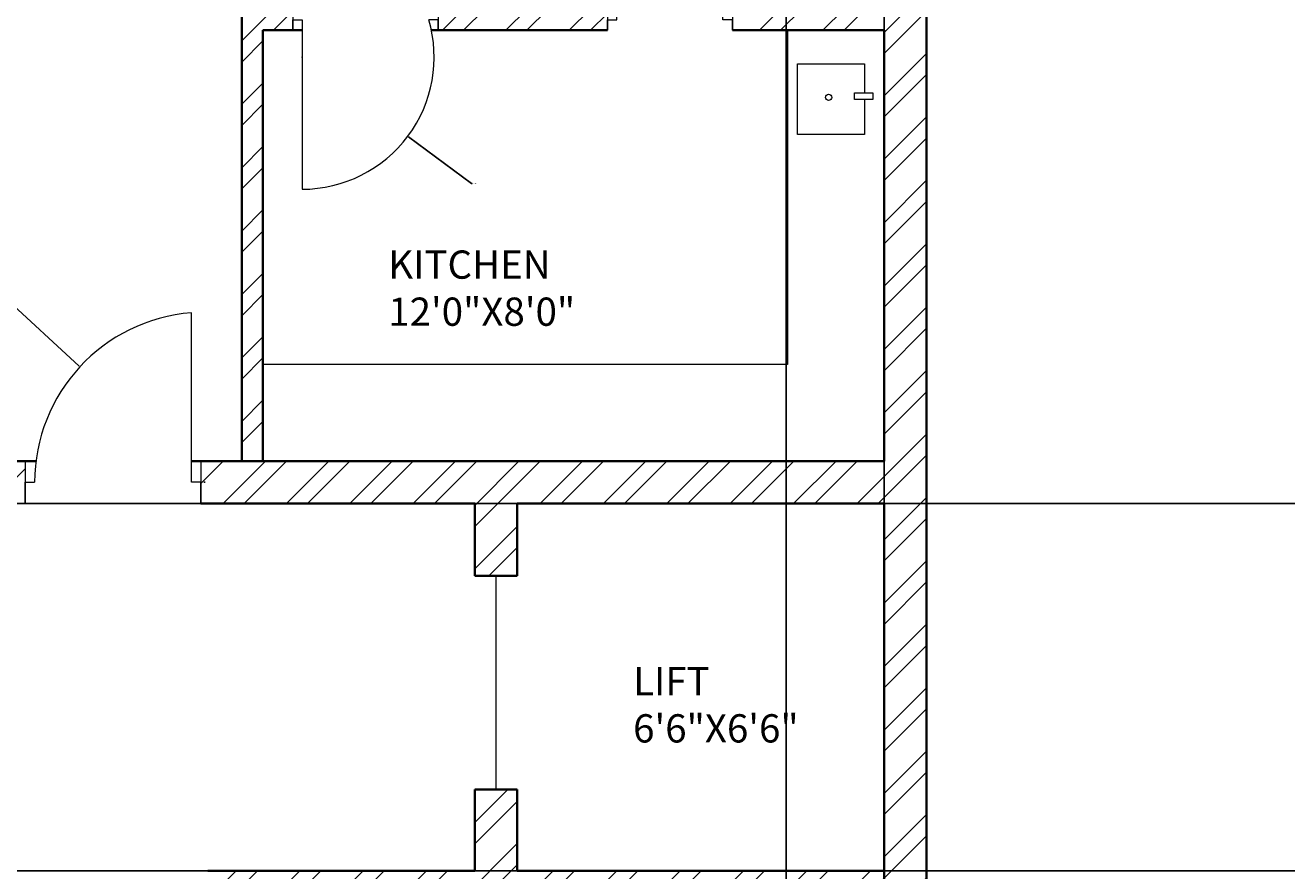
# Model space of a CAD drawing. Units: inches. Extents: x 1355 to 2746, y 1171 to 2751.
# Tile 11 of 24: x 1749 to 2017, y 1686 to 1866. Entities that reach past the tile are written whole.
import ezdxf

# ---------------------------------------------------------------- set-up
doc = ezdxf.new("R2010")
doc.units = ezdxf.units.IN
for name, color, linetype, lineweight in [('A-ANNO-DIMS', 2, 'Continuous', 18), ('A-AREA-IDEN', 7, 'Continuous', 18), ('A-DOOR', 3, 'Continuous', 20), ('A-FLOR-CASE', 30, 'Continuous', 20), ('A-FLOR-FIXT', 9, 'Continuous', 18), ('A-WALL', 7, 'Continuous', 40), ('A-WALL-PATT', 252, 'Continuous', 13)]:
    doc.layers.add(name, color=color, linetype=linetype, lineweight=lineweight)
doc.styles.get("Standard").update_dxf_attribs({"font": 'arial.ttf'})
doc.dimstyles.get("Standard").update_dxf_attribs({"dimtxt": 0.18, "dimasz": 0.18, "dimexe": 0.18, "dimexo": 0.0625, "dimgap": 0.09, "dimtad": 0, "dimtih": 1, "dimtoh": 1, "dimdec": 4, "dimzin": 0, "dimdsep": 46, "dimtxsty": 'Standard', "dimcen": 0.09, "dimadec": 0, "dimazin": 0, "dimtfac": 1, "dimtdec": 4, "dimtofl": 0, "dimtmove": 0, "dimatfit": 3, "dimfxl": 1, "dimtolj": 1, "dimtzin": 0, "dimarcsym": 0})

# ---------------------------------------------------------------- blocks, each defined once
blk = doc.blocks.new('DOOR-ENTRY-N')
for p, q in [((35.29, 4.5), (35.29, 40.5)), ((0, 9), (0, 0)), ((37.29, 9), (37.29, 0)), ((0, 0), (0, 4.5)), ((0, 4.5), (2, 4.5)), ((37.29, 4.5), (35.29, 4.5)), ((37.29, 0), (37.29, 4.5))]:
    blk.add_line(p, q)
blk.add_arc((38.11, 4.5), 36.11, 94.4716, 180)
blk = doc.blocks.new('DOOR-UTILITY-N')
for p, q in [((2, 2.25), (2, 26.25)), ((0, 4.5), (0, 0)), ((26.56, 4.5), (26.56, 0)), ((0, 0), (0, 2.25)), ((0, 2.25), (2, 2.25)), ((26.56, 2.25), (24.56, 2.25)), ((26.56, 0), (26.56, 2.25))]:
    blk.add_line(p, q)
blk.add_arc((0.51, 2.25), 24.05, 0, 86.4557)
blk = doc.blocks.new('DOOR-KITCHEN-N')
for p, q in [((0, 38.25), (0, 33.75)), ((30.9, 38.25), (30.9, 33.75)), ((0, 33.75), (0, 36)), ((0, 36), (2, 36)), ((2, 36), (2, 0)), ((30.9, 36), (28.9, 36)), ((30.9, 33.75), (30.9, 36))]:
    blk.add_line(p, q)
blk.add_arc((2, 28.05), 28.05, 270, 16.4594)
blk = doc.blocks.new('*D102')
at = {"layer": 'A-ANNO-DIMS', "color": 0, "lineweight": -2, "transparency": 16777216}
for p, q in [((2089.33, 1764.3), (1407.53, 1764.3)), ((1407.71, 1764.12), (1407.71, 1725.48)), ((1407.71, 1686.48), (1407.71, 1725.12)), ((2089.33, 1686.3), (1407.53, 1686.3))]:
    blk.add_line(p, q, dxfattribs=at)
at = {"layer": 'A-ANNO-DIMS', "color": 0, "transparency": 16777216}
for points in [[(1407.68, 1764.12), (1407.74, 1764.12), (1407.71, 1764.3)], [(1407.68, 1686.48), (1407.74, 1686.48), (1407.71, 1686.3)]]:
    blk.add_solid(points, dxfattribs=at)
at = {"layer": 'Defpoints', "color": 0, "transparency": 16777216}
for p in [(1407.71, 1764.3), (2089.39, 1764.3), (2089.39, 1686.3)]:
    blk.add_point(p, dxfattribs=at)
at = {"layer": 'A-ANNO-DIMS', "color": 0, "transparency": 16777216, "insert": (1407.71, 1725.3), "char_height": 0.18, "attachment_point": 5}
blk.add_mtext('\\A1;78', dxfattribs=at)
blk = doc.blocks.new('*D103')
at = {"layer": 'A-ANNO-DIMS', "color": 0, "lineweight": -2, "transparency": 16777216}
for p, q in [((2089.33, 1917.3), (1407.53, 1917.3)), ((1407.71, 1917.12), (1407.71, 1840.98)), ((1407.71, 1764.48), (1407.71, 1840.62)), ((2089.33, 1764.3), (1407.53, 1764.3))]:
    blk.add_line(p, q, dxfattribs=at)
at = {"layer": 'A-ANNO-DIMS', "color": 0, "transparency": 16777216}
for points in [[(1407.68, 1917.12), (1407.74, 1917.12), (1407.71, 1917.3)], [(1407.68, 1764.48), (1407.74, 1764.48), (1407.71, 1764.3)]]:
    blk.add_solid(points, dxfattribs=at)
at = {"layer": 'Defpoints', "color": 0, "transparency": 16777216}
for p in [(1407.71, 1917.3), (2089.39, 1917.3), (2089.39, 1764.3)]:
    blk.add_point(p, dxfattribs=at)
at = {"layer": 'A-ANNO-DIMS', "color": 0, "transparency": 16777216, "insert": (1407.71, 1840.8), "char_height": 0.18, "attachment_point": 5}
blk.add_mtext('\\A1;153', dxfattribs=at)
blk = doc.blocks.new('*D107')
at = {"layer": 'A-ANNO-DIMS', "color": 0, "lineweight": -2, "transparency": 16777216}
for p, q in [((2089.33, 1686.3), (1407.53, 1686.3)), ((1407.71, 1686.12), (1407.71, 1622.26)), ((1407.71, 1558.03), (1407.71, 1621.89)), ((2031.09, 1557.85), (1407.53, 1557.85))]:
    blk.add_line(p, q, dxfattribs=at)
at = {"layer": 'A-ANNO-DIMS', "color": 0, "transparency": 16777216}
for points in [[(1407.68, 1686.12), (1407.74, 1686.12), (1407.71, 1686.3)], [(1407.68, 1558.03), (1407.74, 1558.03), (1407.71, 1557.85)]]:
    blk.add_solid(points, dxfattribs=at)
at = {"layer": 'Defpoints', "color": 0, "transparency": 16777216}
for p in [(1407.71, 1686.3), (2089.39, 1686.3), (2031.15, 1557.85)]:
    blk.add_point(p, dxfattribs=at)
at = {"layer": 'A-ANNO-DIMS', "color": 0, "transparency": 16777216, "insert": (1407.71, 1622.07), "char_height": 0.18, "attachment_point": 5}
blk.add_mtext('\\A1;128.46', dxfattribs=at)
blk = doc.blocks.new('*D145')
at = {"layer": 'A-ANNO-DIMS', "color": 0, "lineweight": -2, "transparency": 16777216}
for p, q in [((1910.88, 1399.86), (1910.88, 2716.58)), ((1911.06, 2716.4), (1920.83, 2716.4)), ((1931.53, 2716.4), (1921.76, 2716.4)), ((1931.71, 1399.86), (1931.71, 2716.58))]:
    blk.add_line(p, q, dxfattribs=at)
at = {"layer": 'A-ANNO-DIMS', "color": 0, "transparency": 16777216}
for points in [[(1911.06, 2716.43), (1911.06, 2716.37), (1910.88, 2716.4)], [(1931.53, 2716.43), (1931.53, 2716.37), (1931.71, 2716.4)]]:
    blk.add_solid(points, dxfattribs=at)
at = {"layer": 'Defpoints', "color": 0, "transparency": 16777216}
for p in [(1931.71, 2716.4), (1910.88, 1399.8), (1931.71, 1399.8)]:
    blk.add_point(p, dxfattribs=at)
at = {"layer": 'A-ANNO-DIMS', "color": 0, "transparency": 16777216, "insert": (1921.3, 2716.4), "char_height": 0.18, "attachment_point": 5}
blk.add_mtext('\\A1;20.824', dxfattribs=at)
blk = doc.blocks.new('*D154')
at = {"layer": 'A-ANNO-DIMS', "color": 0, "lineweight": -2, "transparency": 16777216}
for p, q in [((1744.73, 1808.03), (1744.91, 1808.03)), ((1744.91, 1808.03), (1760.69, 1793.44)), ((1787.24, 1768.8), (1787.42, 1768.8)), ((1787.33, 1768.71), (1787.33, 1768.89))]:
    blk.add_line(p, q, dxfattribs=at)
at = {"layer": 'A-ANNO-DIMS', "color": 0, "transparency": 16777216}
blk.add_solid([(1760.71, 1793.46), (1760.67, 1793.42), (1760.82, 1793.32)], dxfattribs=at)
at = {"layer": 'Defpoints', "color": 0, "transparency": 16777216}
for p in [(1760.82, 1793.32), (1787.33, 1768.8)]:
    blk.add_point(p, dxfattribs=at)
at = {"layer": 'A-ANNO-DIMS', "color": 0, "transparency": 16777216, "insert": (1744.27, 1808.03), "char_height": 0.18, "attachment_point": 5}
blk.add_mtext('\\A1;R36.11', dxfattribs=at)
blk = doc.blocks.new('*D158')
at = {"layer": 'A-ANNO-DIMS', "color": 0, "lineweight": -2, "transparency": 16777216}
for p, q in [((1807.96, 1859.1), (1808.14, 1859.1)), ((1808.05, 1859.01), (1808.05, 1859.19)), ((1844.01, 1832.24), (1830.67, 1842.2)), ((1844.19, 1832.24), (1844.01, 1832.24))]:
    blk.add_line(p, q, dxfattribs=at)
at = {"layer": 'A-ANNO-DIMS', "color": 0, "transparency": 16777216}
blk.add_solid([(1830.69, 1842.23), (1830.65, 1842.18), (1830.52, 1842.31)], dxfattribs=at)
at = {"layer": 'Defpoints', "color": 0, "transparency": 16777216}
for p in [(1808.05, 1859.1), (1830.52, 1842.31)]:
    blk.add_point(p, dxfattribs=at)
at = {"layer": 'A-ANNO-DIMS', "color": 0, "transparency": 16777216, "insert": (1844.67, 1832.24), "char_height": 0.18, "attachment_point": 5}
blk.add_mtext('\\A1;R28.05', dxfattribs=at)

msp = doc.modelspace()

# ---------------------------------------------------------------- hatches: boundary and pattern name
at = {"layer": 'A-WALL-PATT'}
h = msp.add_hatch(dxfattribs=at)
h.set_pattern_fill('ANSI32', color=256)
h.paths.add_polyline_path([(1660.2083, 2139.3018), (1614.5977, 2139.3018), (1614.5977, 2130.3018), (1655.7083, 2130.3018), (1655.7083, 1981.8018), (1660.2083, 1981.8018), (1660.2083, 2090.7225), (1692.5832, 2090.7225), (1692.5832, 2095.2225), (1660.2083, 2095.2225)])
h.paths.add_polyline_path([(1523.7083, 2130.3018), (1554.5977, 2130.3018), (1554.5977, 2134.8018), (1554.5977, 2139.3018), (1514.7083, 2139.3018), (1514.7083, 2071.8385), (1523.7083, 2071.8385)])
h.paths.add_polyline_path([(1940.7083, 2139.3018), (1883.7928, 2139.3018), (1883.7928, 2130.3018), (1931.7083, 2130.3018), (1931.7083, 2098.3333), (1940.7083, 2098.3333)])
h.paths.add_polyline_path([(1799.7083, 2130.3018), (1823.7928, 2130.3018), (1823.7928, 2134.8018), (1823.7928, 2139.3018), (1795.2083, 2139.3018), (1795.2083, 2130.3018), (1795.2083, 2095.2225), (1759.2134, 2095.2225), (1759.2134, 2090.7225), (1795.2083, 2090.7225), (1795.2083, 1981.8018), (1799.7083, 1981.8018), (1799.7083, 1986.3018)])
h.paths.add_polyline_path([(1940.7083, 2038.3333), (1931.7083, 2038.3333), (1931.7083, 1986.3018), (1832.7083, 1986.3018), (1832.7083, 1947.1338), (1837.2083, 1947.1338), (1837.2083, 1981.8018), (1931.7083, 1981.8018), (1931.7083, 1967.1939), (1940.7083, 1967.1939)])
h.paths.add_polyline_path([(1940.7083, 1943.1939), (1931.7083, 1943.1939), (1931.7083, 1921.8018), (1837.2083, 1921.8018), (1837.2083, 1926.0511), (1832.7083, 1926.0511), (1832.7083, 1917.3018), (1931.7083, 1917.3018), (1931.7083, 1908.3321), (1940.7083, 1908.3321)])
h.paths.add_polyline_path([(1940.7083, 1884.3321), (1931.7083, 1884.3321), (1931.7083, 1869.3018), (1899.4583, 1869.3018), (1899.4583, 1864.8018), (1931.7083, 1864.8018), (1931.7083, 1773.3018), (1786.5143, 1773.3018), (1786.5143, 1764.3018), (1844.7083, 1764.3018), (1844.7083, 1748.9343), (1853.7083, 1748.9343), (1853.7083, 1764.3018), (1931.7083, 1764.3018), (1931.7083, 1652.9424), (1940.7083, 1652.9424)])
h.paths.add_polyline_path([(1799.7083, 1864.8018), (1806.0522, 1864.8018), (1806.0522, 1867.0518), (1806.0522, 1869.3018), (1799.7083, 1869.3018), (1799.7083, 1917.3018), (1799.7083, 1921.8018), (1795.2083, 1921.8018), (1795.2083, 1773.3018), (1799.7083, 1773.3018)])
h.paths.add_polyline_path([(1872.8988, 1867.0518), (1872.8988, 1869.3018), (1867.2083, 1869.3018), (1867.2083, 1917.3018), (1862.7083, 1917.3018), (1862.7083, 1869.3018), (1836.9546, 1869.3018), (1836.9546, 1864.8018), (1862.7083, 1864.8018), (1872.8988, 1864.8018)])
h.paths.add_polyline_path([(1749.2197, 1773.3018), (1655.7083, 1773.3018), (1523.7083, 1773.3018), (1523.7083, 1828.4963), (1514.7083, 1828.4963), (1514.7083, 1753.9033), (1519.2083, 1753.9033), (1523.7083, 1753.9033), (1523.7083, 1764.3018), (1655.7083, 1764.3018), (1749.2197, 1764.3018), (1749.2197, 1768.8018)])
h.paths.add_polyline_path([(1660.2083, 1921.8018), (1655.7083, 1921.8018), (1655.7083, 1917.3018), (1655.7083, 1773.3018), (1660.2083, 1773.3018)])
h.paths.add_polyline_path([(1523.7083, 2011.8385), (1514.7083, 2011.8385), (1514.7083, 1973.114), (1519.2083, 1973.114), (1523.7083, 1973.114), (1523.7083, 1976.8227), (1523.7083, 1981.8018), (1618.2083, 1981.8018), (1618.2083, 1921.8018), (1553.707, 1921.8018), (1553.707, 1917.3018), (1622.7083, 1917.3018), (1622.7083, 1919.5518), (1622.7083, 1921.8018), (1622.7083, 1986.3018), (1523.7083, 1986.3018)])
h.paths.add_polyline_path([(1529.6686, 1919.5518), (1529.6686, 1921.8018), (1523.7083, 1921.8018), (1523.7083, 1949.114), (1514.7083, 1949.114), (1514.7083, 1888.4963), (1523.7083, 1888.4963), (1523.7083, 1917.3018), (1529.6686, 1917.3018)])
h.paths.add_polyline_path([(1538.9419, 1775.643), (1585.5504, 1775.643), (1585.5504, 1798.0318), (1538.9419, 1798.0318)], flags=25)
h.paths.add_polyline_path([(1696.7097, 1497.3356), (1769.5651, 1497.3356), (1769.5651, 1523.4559), (1696.7097, 1523.4559)], flags=9)
h.paths.add_polyline_path([(1629.1643, 1230.5133), (1877.0879, 1230.5133), (1877.0879, 1267.606), (1629.1643, 1267.606)], flags=9)
h.paths.add_polyline_path([(2533.4462, 2215.4033), (2579.9292, 2215.4033), (2579.9292, 2231.889), (2533.4462, 2231.889)], flags=9)
h.paths.add_polyline_path([(2540.822, 2515.6945), (2594.2245, 2515.6945), (2594.2245, 2545.5463), (2540.822, 2545.5463)], flags=9)
h.paths.add_polyline_path([(2535.9857, 2588.2819), (2582.4687, 2588.2819), (2582.4687, 2604.7675), (2535.9857, 2604.7675)], flags=9)
h.paths.add_polyline_path([(2537.1627, 2617.1172), (2649.1245, 2617.1172), (2649.1245, 2633.6029), (2537.1627, 2633.6029)], flags=9)
h.paths.add_polyline_path([(2218.0051, 2168.228), (2363.9573, 2168.228), (2363.9573, 2205.3208), (2218.0051, 2205.3208)], flags=9)
h.paths.add_polyline_path([(1650.2156, 2165.3631), (1800.3547, 2165.3631), (1800.3547, 2202.4559), (1650.2156, 2202.4559)], flags=9)
h.paths.add_polyline_path([(2553.9592, 1610.7663), (2588.4203, 1610.7663), (2588.4203, 1660.2233), (2553.9592, 1660.2233)], flags=9)
h.paths.add_polyline_path([(1549.0868, 1648.2033), (1595.6952, 1648.2033), (1595.6952, 1670.5921), (1549.0868, 1670.5921)], flags=9)
h.paths.add_polyline_path([(1546.9525, 1502.0931), (1583.3413, 1502.0931), (1583.3413, 1524.4819), (1546.9525, 1524.4819)], flags=9)
h.paths.add_polyline_path([(1540.7704, 1433.4431), (1587.3788, 1433.4431), (1587.3788, 1455.8319), (1540.7704, 1455.8319)], flags=9)
h.paths.add_polyline_path([(1683.6524, 1321.5269), (1760.6169, 1321.5269), (1760.6169, 1333.8911), (1683.6524, 1333.8911)], flags=9)
h.paths.add_polyline_path([(1832.0485, 1356.0874), (1873.0989, 1356.0874), (1873.0989, 1378.4762), (1832.0485, 1378.4762)], flags=9)
h.paths.add_polyline_path([(1877.9694, 1431.2138), (1926.3827, 1431.2138), (1926.3827, 1453.578), (1877.9694, 1453.578)], flags=9)
h.paths.add_polyline_path([(1847.3106, 1499.8371), (1883.6994, 1499.8371), (1883.6994, 1522.2259), (1847.3106, 1522.2259)], flags=9)
h.paths.add_polyline_path([(1813.7015, 1640.7287), (1860.3099, 1640.7287), (1860.3099, 1663.1175), (1813.7015, 1663.1175)], flags=9)
h.paths.add_polyline_path([(1876.2576, 1710.2471), (1912.9452, 1710.2471), (1912.9452, 1732.6359), (1876.2576, 1732.6359)], flags=25)
h.paths.add_polyline_path([(1695.9163, 1715.3064), (1736.9668, 1715.3064), (1736.9668, 1737.6952), (1695.9163, 1737.6952)], flags=9)
h.paths.add_polyline_path([(1881.8583, 1888.9094), (1930.2717, 1888.9094), (1930.2717, 1911.2737), (1881.8583, 1911.2737)], flags=9)
h.paths.add_polyline_path([(1823.9298, 1798.6431), (1864.9803, 1798.6431), (1864.9803, 1821.0319), (1823.9298, 1821.0319)], flags=25)
h.paths.add_polyline_path([(1845.6062, 1948.1408), (1881.995, 1948.1408), (1881.995, 1970.5296), (1845.6062, 1970.5296)], flags=25)
h.paths.add_polyline_path([(1849.027, 1991.5151), (1895.6355, 1991.5151), (1895.6355, 2013.9039), (1849.027, 2013.9039)], flags=25)
h.paths.add_polyline_path([(1684.9725, 2113.8416), (1764.2658, 2113.8416), (1764.2658, 2126.2058), (1684.9725, 2126.2058)], flags=9)
h.paths.add_polyline_path([(1688.6193, 1913.0676), (1776.2005, 1913.0676), (1776.2005, 1935.4564), (1688.6193, 1935.4564)], flags=9)
h.paths.add_polyline_path([(1571.4689, 1930.9816), (1607.8577, 1930.9816), (1607.8577, 1953.3704), (1571.4689, 1953.3704)], flags=25)
h.paths.add_polyline_path([(1535.3581, 1998.3125), (1581.9665, 1998.3125), (1581.9665, 2020.7014), (1535.3581, 2020.7014)], flags=9)
h = msp.add_hatch(dxfattribs=at)
h.set_pattern_fill('ANSI32', color=256)
h.paths.add_polyline_path([(1749.2197, 1686.3018), (1732.6892, 1686.3018), (1523.7083, 1686.3018), (1523.7083, 1705.9033), (1514.7083, 1705.9033), (1514.7083, 1647.8732), (1519.2083, 1647.8732), (1523.7083, 1647.8732), (1523.7083, 1677.3018), (1655.7083, 1677.3018), (1655.7083, 1528.8018), (1660.2083, 1528.8018), (1660.2083, 1677.3018), (1732.6892, 1677.3018), (1749.2197, 1677.3018)])
h.paths.add_polyline_path([(1931.7083, 1686.3018), (1853.7083, 1686.3018), (1853.7083, 1703.5696), (1844.7083, 1703.5696), (1844.7083, 1686.3018), (1788.0274, 1686.3018), (1788.0274, 1677.3018), (1795.2083, 1677.3018), (1795.2083, 1528.8018), (1799.7083, 1528.8018), (1799.7083, 1677.3018), (1844.7083, 1677.3018), (1931.7083, 1677.3018)])
h.paths.add_polyline_path([(1931.7083, 1533.3018), (1844.7083, 1533.3018), (1832.7083, 1533.3018), (1832.7083, 1531.0518), (1832.7083, 1528.8018), (1832.7083, 1495.7519), (1837.2083, 1495.7519), (1837.2083, 1528.8018), (1931.7083, 1528.8018)])
h.paths.add_polyline_path([(1940.7083, 1592.9424), (1931.7083, 1592.9424), (1931.7083, 1506.7845), (1940.7083, 1506.7845)])
h.paths.add_polyline_path([(1940.7083, 1482.7845), (1936.2083, 1482.7845), (1931.7083, 1482.7845), (1931.7083, 1320.3018), (1880.7083, 1320.3018), (1880.7083, 1311.3018), (1940.7083, 1311.3018)])
h.paths.add_polyline_path([(1931.7083, 1468.8018), (1844.7083, 1468.8018), (1837.2083, 1468.8018), (1837.2083, 1474.34), (1832.7083, 1474.34), (1832.7083, 1468.8018), (1832.7083, 1464.3018), (1844.7083, 1464.3018), (1931.7083, 1464.3018)])
h.paths.add_polyline_path([(1863.8571, 1464.3018), (1859.3571, 1464.3018), (1859.3571, 1404.1662), (1838.1542, 1404.1662), (1838.1542, 1399.8018), (1869.4185, 1399.8018), (1869.4185, 1402.0518), (1869.4185, 1404.3018), (1863.8571, 1404.3018)])
h.paths.add_polyline_path([(1799.7083, 1399.6662), (1805.4082, 1399.6662), (1805.4082, 1401.9162), (1805.4082, 1404.1662), (1799.7083, 1404.1662), (1799.7083, 1464.3018), (1799.7083, 1468.8018), (1795.2083, 1468.8018), (1795.2083, 1356.2098), (1761.2597, 1356.2098), (1761.2597, 1351.7098), (1795.2083, 1351.7098), (1795.2083, 1320.3018), (1795.2083, 1311.3018), (1844.7083, 1311.3018), (1844.7083, 1315.8018), (1844.7083, 1320.3018), (1799.7083, 1320.3018)])
h.paths.add_polyline_path([(1692.9218, 1356.2098), (1660.2083, 1356.2098), (1660.2083, 1430.786), (1657.9583, 1430.786), (1655.7083, 1430.786), (1655.7083, 1320.3018), (1611.934, 1320.3018), (1611.934, 1311.3018), (1660.2083, 1311.3018), (1660.2083, 1351.7098), (1692.9218, 1351.7098)])
h.paths.add_polyline_path([(1523.7083, 1372.653), (1514.7083, 1372.653), (1514.7083, 1311.3018), (1551.934, 1311.3018), (1551.934, 1315.8018), (1551.934, 1320.3018), (1523.7083, 1320.3018)])
h.paths.add_polyline_path([(1523.7083, 1490.9023), (1514.7083, 1490.9023), (1514.7083, 1432.653), (1519.2083, 1432.653), (1523.7083, 1432.653)])
h.paths.add_polyline_path([(1660.2083, 1468.8018), (1622.7083, 1468.8018), (1622.7083, 1473.1566), (1618.2083, 1473.1566), (1618.2083, 1468.8018), (1523.7083, 1468.8018), (1523.7083, 1464.3018), (1655.7083, 1464.3018), (1655.7083, 1460.5634), (1660.2083, 1460.5634)])
h.paths.add_polyline_path([(1523.7083, 1587.8732), (1514.7083, 1587.8732), (1514.7083, 1514.9023), (1519.2083, 1514.9023), (1523.7083, 1514.9023)])
h.paths.add_polyline_path([(1622.7083, 1533.3018), (1523.7083, 1533.3018), (1523.7083, 1528.8018), (1618.2083, 1528.8018), (1618.2083, 1494.4205), (1622.7083, 1494.4205), (1622.7083, 1528.8018)])
h.paths.add_polyline_path([(1696.7097, 1497.3356), (1769.5651, 1497.3356), (1769.5651, 1523.4559), (1696.7097, 1523.4559)], flags=9)
h.paths.add_polyline_path([(1629.1643, 1230.5133), (1877.0879, 1230.5133), (1877.0879, 1267.606), (1629.1643, 1267.606)], flags=9)
h.paths.add_polyline_path([(2533.4462, 2215.4033), (2579.9292, 2215.4033), (2579.9292, 2231.889), (2533.4462, 2231.889)], flags=9)
h.paths.add_polyline_path([(2540.822, 2515.6945), (2594.2245, 2515.6945), (2594.2245, 2545.5463), (2540.822, 2545.5463)], flags=9)
h.paths.add_polyline_path([(2535.9857, 2588.2819), (2582.4687, 2588.2819), (2582.4687, 2604.7675), (2535.9857, 2604.7675)], flags=9)
h.paths.add_polyline_path([(2537.1627, 2617.1172), (2649.1245, 2617.1172), (2649.1245, 2633.6029), (2537.1627, 2633.6029)], flags=9)
h.paths.add_polyline_path([(2218.0051, 2168.228), (2363.9573, 2168.228), (2363.9573, 2205.3208), (2218.0051, 2205.3208)], flags=9)
h.paths.add_polyline_path([(1650.2156, 2165.3631), (1800.3547, 2165.3631), (1800.3547, 2202.4559), (1650.2156, 2202.4559)], flags=9)
h.paths.add_polyline_path([(2553.9592, 1610.7663), (2588.4203, 1610.7663), (2588.4203, 1660.2233), (2553.9592, 1660.2233)], flags=9)
h.paths.add_polyline_path([(1549.0868, 1648.2033), (1595.6952, 1648.2033), (1595.6952, 1670.5921), (1549.0868, 1670.5921)], flags=25)
h.paths.add_polyline_path([(1546.9525, 1502.0931), (1583.3413, 1502.0931), (1583.3413, 1524.4819), (1546.9525, 1524.4819)], flags=25)
h.paths.add_polyline_path([(1540.7704, 1433.4431), (1587.3788, 1433.4431), (1587.3788, 1455.8319), (1540.7704, 1455.8319)], flags=9)
h.paths.add_polyline_path([(1683.6524, 1321.5269), (1760.6169, 1321.5269), (1760.6169, 1333.8911), (1683.6524, 1333.8911)], flags=9)
h.paths.add_polyline_path([(1832.0485, 1356.0874), (1873.0989, 1356.0874), (1873.0989, 1378.4762), (1832.0485, 1378.4762)], flags=9)
h.paths.add_polyline_path([(1877.9694, 1431.2138), (1926.3827, 1431.2138), (1926.3827, 1453.578), (1877.9694, 1453.578)], flags=9)
h.paths.add_polyline_path([(1847.3106, 1499.8371), (1883.6994, 1499.8371), (1883.6994, 1522.2259), (1847.3106, 1522.2259)], flags=25)
h.paths.add_polyline_path([(1813.7015, 1640.7287), (1860.3099, 1640.7287), (1860.3099, 1663.1175), (1813.7015, 1663.1175)], flags=25)
h.paths.add_polyline_path([(1876.2576, 1710.2471), (1912.9452, 1710.2471), (1912.9452, 1732.6359), (1876.2576, 1732.6359)], flags=9)
h.paths.add_polyline_path([(1695.9163, 1715.3064), (1736.9668, 1715.3064), (1736.9668, 1737.6952), (1695.9163, 1737.6952)], flags=9)
h.paths.add_polyline_path([(1881.8583, 1888.9094), (1930.2717, 1888.9094), (1930.2717, 1911.2737), (1881.8583, 1911.2737)], flags=9)
h.paths.add_polyline_path([(1823.9298, 1798.6431), (1864.9803, 1798.6431), (1864.9803, 1821.0319), (1823.9298, 1821.0319)], flags=9)
h.paths.add_polyline_path([(1845.6062, 1948.1408), (1881.995, 1948.1408), (1881.995, 1970.5296), (1845.6062, 1970.5296)], flags=9)
h.paths.add_polyline_path([(1849.027, 1991.5151), (1895.6355, 1991.5151), (1895.6355, 2013.9039), (1849.027, 2013.9039)], flags=9)
h.paths.add_polyline_path([(1684.9725, 2113.8416), (1764.2658, 2113.8416), (1764.2658, 2126.2058), (1684.9725, 2126.2058)], flags=9)
h.paths.add_polyline_path([(1688.6193, 1913.0676), (1776.2005, 1913.0676), (1776.2005, 1935.4564), (1688.6193, 1935.4564)], flags=9)
h.paths.add_polyline_path([(1538.9419, 1775.643), (1585.5504, 1775.643), (1585.5504, 1798.0318), (1538.9419, 1798.0318)], flags=9)
h.paths.add_polyline_path([(1571.4689, 1930.9816), (1607.8577, 1930.9816), (1607.8577, 1953.3704), (1571.4689, 1953.3704)], flags=9)
h.paths.add_polyline_path([(1535.3581, 1998.3125), (1581.9665, 1998.3125), (1581.9665, 2020.7014), (1535.3581, 2020.7014)], flags=9)

# ---------------------------------------------------------------- linework, layer by layer
at = {"layer": 'A-DOOR'}
msp.add_line((1849.2083, 1748.9343), (1849.2083, 1703.5696), dxfattribs=at)
at = {"layer": 'A-FLOR-CASE'}
for p, q in [((1911.1891, 1864.8018), (1911.1891, 1793.8497)), ((1911.1891, 1793.8497), (1799.7083, 1793.8497))]:
    msp.add_line(p, q, dxfattribs=at)
at = {"layer": 'A-FLOR-FIXT'}
msp.add_lwpolyline([(1927.5317, 1850.1078), (1927.5317, 1842.6761), (1913.3259, 1842.6761), (1913.3259, 1857.709), (1927.5317, 1857.709), (1927.5317, 1851.5305)], dxfattribs=at)
msp.add_lwpolyline([(1925.392, 1851.5305), (1929.2822, 1851.5305), (1929.2822, 1850.1078), (1925.392, 1850.1078)], close=True, dxfattribs=at)
msp.add_circle((1919.9125, 1850.5584), 0.6639, dxfattribs=at)
at = {"layer": 'A-WALL'}
for p, q in [((1940.7083, 2139.3018), (1940.7083, 1311.3018)), ((1795.2083, 1921.8018), (1795.2083, 1773.3018)), ((1799.7083, 1864.8018), (1808.0522, 1864.8018)), ((1799.7083, 1864.8018), (1799.7083, 1773.3018)), ((1835.5193, 1864.8018), (1862.7083, 1864.8018)), ((1862.7083, 1864.8018), (1872.8988, 1864.8018)), ((1899.4583, 1864.8018), (1931.7083, 1864.8018)), ((1931.7083, 1864.8018), (1931.7083, 1773.3018)), ((1655.7083, 1773.3018), (1751.5012, 1773.3018)), ((1784.5143, 1773.3018), (1931.7083, 1773.3018)), ((1786.5143, 1764.3018), (1844.7083, 1764.3018)), ((1844.7083, 1764.3018), (1844.7083, 1748.9343)), ((1853.7083, 1764.3018), (1853.7083, 1748.9343)), ((1853.7083, 1764.3018), (1931.7083, 1764.3018)), ((1931.7083, 1764.3018), (1931.7083, 1320.3018)), ((1844.7083, 1748.9343), (1853.7083, 1748.9343)), ((1844.7083, 1703.5696), (1853.7083, 1703.5696)), ((1844.7083, 1703.5696), (1844.7083, 1686.3018)), ((1853.7083, 1703.5696), (1853.7083, 1686.3018)), ((1844.7083, 1686.3018), (1788.0274, 1686.3018)), ((1853.7083, 1686.3018), (1931.7083, 1686.3018))]:
    msp.add_line(p, q, dxfattribs=at)

# ---------------------------------------------------------------- block references
at = {"layer": 'A-DOOR'}
for name, p in [('DOOR-UTILITY-N', (1872.899, 1864.802)), ('DOOR-KITCHEN-N', (1806.052, 1831.052)), ('DOOR-ENTRY-N', (1749.22, 1764.302))]:
    msp.add_blockref(name, p, dxfattribs=at)

# ---------------------------------------------------------------- texts
at = {"layer": 'A-AREA-IDEN', "char_height": 6, "attachment_point": 1}
for s, width, insert in [('KITCHEN\\P12\'0"X8\'0"', 74.562966, (1826.3425, 1818.0462)), ('LIFT\\P6\'6"X6\'6"', 62.336771, (1878.3715, 1729.5479))]:
    msp.add_mtext_dynamic_manual_height_columns(s, width=width, gutter_width=12.5, heights=[0], dxfattribs=dict(at, insert=insert))

# ---------------------------------------------------------------- dimensions: what is measured, and where the dimension line sits
at = {"layer": 'A-ANNO-DIMS'}
dim = msp.add_linear_dim(base=(1931.7083, 2716.3999), p1=(1910.8842, 1399.8018), p2=(1931.7083, 1399.8018), dimstyle='Standard', override={"dimdec": 3, "dimlfac": 1, "dimrnd": 0, "dimzin": 0, "dimdsep": 46, "dimlunit": 2}, dxfattribs=at)
dim.commit()
dim.dimension.update_dxf_attribs({"geometry": '*D145', "text_midpoint": (1921.2962, 2716.3999)})
for base, p1, p2, override, picture, middle in [((1407.7083, 1917.3018), (2089.3909, 1764.3018), (2089.3909, 1917.3018), {"dimdec": 0, "dimlfac": 1, "dimrnd": 0, "dimzin": 0, "dimdsep": 46, "dimlunit": 2}, '*D103', (1407.7083, 1840.8018)), ((1407.7083, 1764.3018), (2089.3909, 1686.3018), (2089.3909, 1764.3018), {"dimdec": 0, "dimlfac": 1, "dimrnd": 0, "dimzin": 0, "dimdsep": 46, "dimlunit": 2}, '*D102', (1407.7083, 1725.3018)), ((1407.7083, 1686.3018), (2031.1535, 1557.845), (2089.3909, 1686.3018), {"dimdec": 2, "dimlfac": 1, "dimrnd": 0, "dimzin": 0, "dimdsep": 46, "dimlunit": 2}, '*D107', (1407.7083, 1622.0734))]:
    dim = msp.add_linear_dim(base=base, p1=p1, p2=p2, angle=90, dimstyle='Standard', override=override, dxfattribs=at)
    dim.commit()
    dim.dimension.update_dxf_attribs({"geometry": picture, "text_midpoint": middle})
for center, mpoint, picture, middle in [((1808.0522, 1859.1037), (1830.5232, 1842.3119), '*D158', (1844.6662, 1832.2368)), ((1787.3297, 1768.8018), (1760.8193, 1793.3197), '*D154', (1744.2706, 1808.0305))]:
    dim = msp.add_radius_dim(center=center, mpoint=mpoint, dimstyle='Standard', override={"dimdec": 2, "dimlfac": 1, "dimrnd": 0, "dimzin": 0, "dimdsep": 46, "dimlunit": 2}, dxfattribs=at)
    dim.commit()
    dim.dimension.update_dxf_attribs({"geometry": picture, "text_midpoint": middle, "dimtype": 164})

doc.saveas('drawing.dxf')
